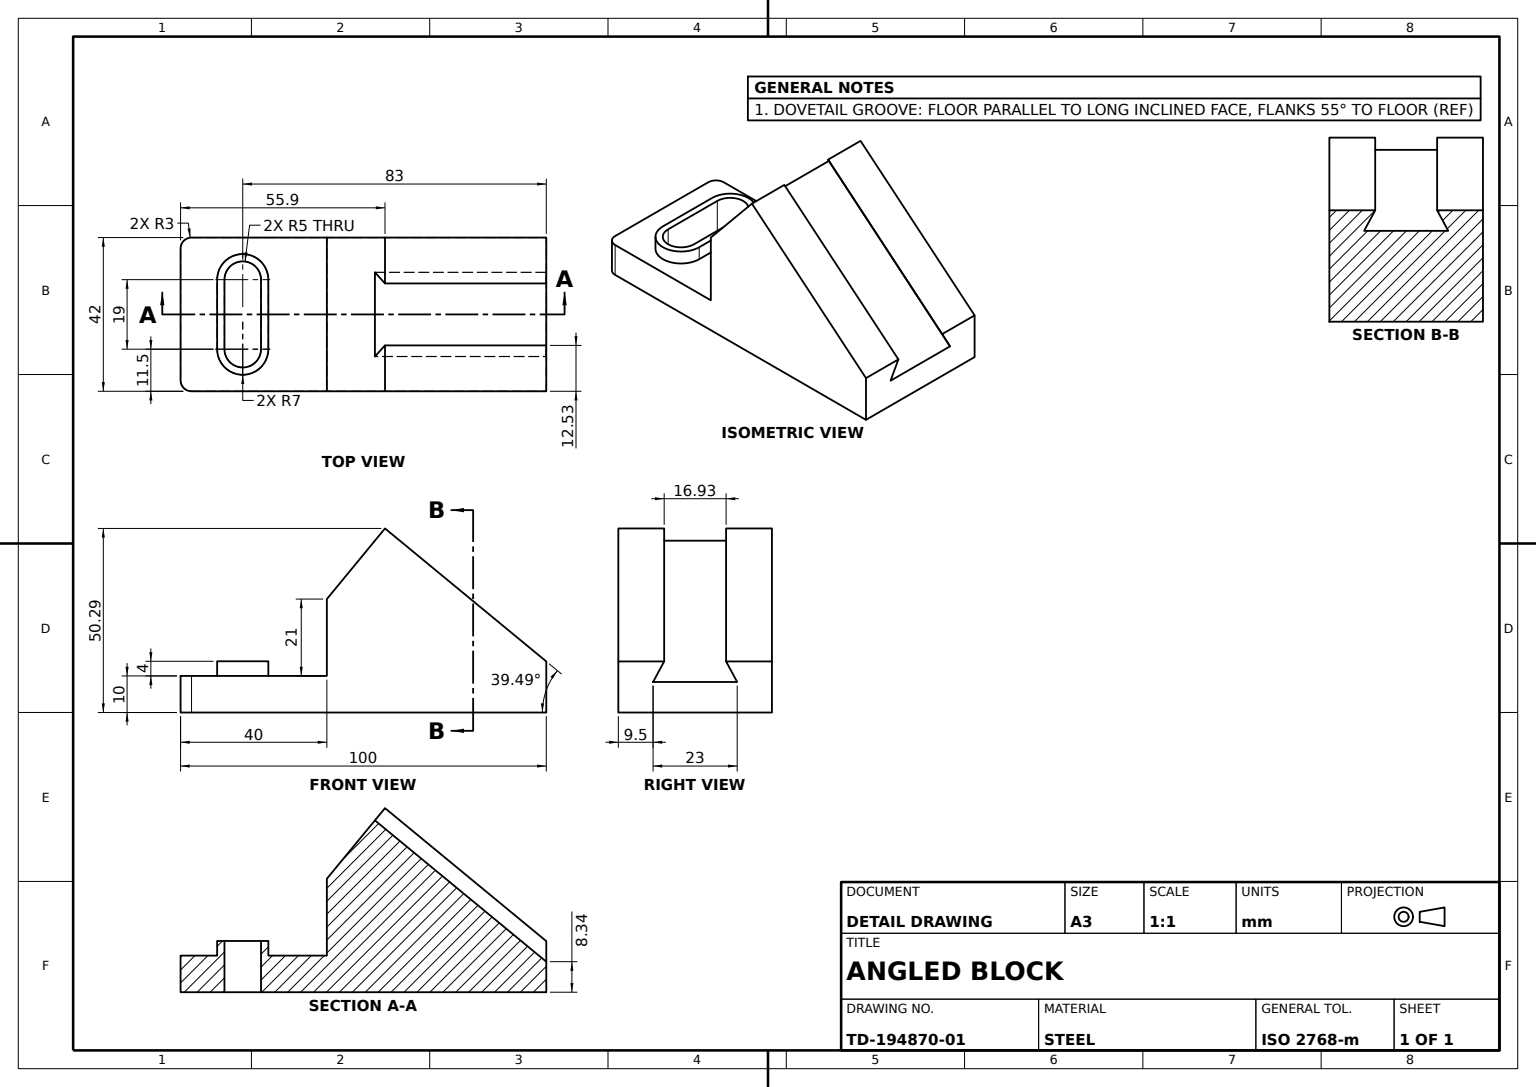
SolidWorks part; units mm, degrees
material "Plain Carbon Steel"
ref_plane "Front Plane" through (0, 0, 0) normal (0, 0, 1) x (1, 0, 0)
ref_plane "Top Plane" through (0, 0, 0) normal (0, 1, 0) x (1, 0, 0)
ref_plane "Right Plane" through (0, 0, 0) normal (1, 0, 0) x (0, 0, -1)
sketch "Base Profile Sketch" plane through (0, 0, 0) normal (0, 0, 1) x (1, 0, 0)
  line L0 (0, 0) -> (-100, 0)
  line L1 (-100, 0) -> (-100, 10)
  line L2 (-100, 10) -> (-60, 10)
  line L3 (-60, 10) -> (-60, 31)
  line L4 (-60, 31) -> (-44.1027, 50.2945)
  line L5 (-44.1027, 50.2945) -> (0, 22.736)
  line L6 (0, 22.736) -> (0, 0)
  dimension "D1" = 60
  dimension "D2" = 22.736
  dimension "D3" = 25
  dimension "D4" = 31
  dimension "D5" = 100
  dimension "D6" = 10
  dimension "D7" = 55.8973
extrude "Base Block" add sketch "Base Profile Sketch" along normal mid plane 42
sketch "Slot Boss Sketch" plane through (0, 10, 0) normal (0, 1, 0) x (1, 0, 0)
  line L0 (-88, 9.5) -> (-88, -9.5)
  line L4 (-90, 9.5) -> (-90, -9.5)
  line L5 (-76, 9.5) -> (-76, -9.5)
  line L6 (-78, 9.5) -> (-78, -9.5)
  arc A0 (-76, 9.5) -> (-90, 9.5) centre (-83, 9.5) ccw
  arc A1 (-90, -9.5) -> (-76, -9.5) centre (-83, -9.5) ccw
  arc A2 (-78, 9.5) -> (-88, 9.5) centre (-83, 9.5) ccw
  arc A3 (-88, -9.5) -> (-78, -9.5) centre (-83, -9.5) ccw
  dimension "D2" = 14
  dimension "D3" = 14
  dimension "D1" = 2
  dimension "D4" = 19
  dimension "D5" = 83
  dimension "D6" = 9.5
extrude "Slot Boss" add sketch "Slot Boss Sketch" along normal blind 4
sketch "Mounting Slot Sketch" plane through (0, 10, 0) normal (0, 1, 0) x (1, 0, 0)
  line L0 (-88, 9.5) -> (-88, -9.5)
  line L1 (-78, 9.5) -> (-78, -9.5)
  arc A0 (-78, 9.5) -> (-88, 9.5) centre (-83, 9.5) ccw
  arc A1 (-88, -9.5) -> (-78, -9.5) centre (-83, -9.5) ccw
extrude "Mounting Slot" cut sketch "Mounting Slot Sketch" against normal blind 34
sketch "Dovetail Groove Sketch" plane through (-50.9523, 41.9811, 0) normal (-0.7718, 0.6359, 0) x (0, 0, 1)
  line L0 (-11.5, 6.439) -> (-8.4663, 10.7717)
  line L2 (-11.5, 6.439) -> (11.5, 6.439)
  line L3 (11.5, 6.439) -> (8.4663, 10.7717)
  line L5 (-8.4663, 10.7717) -> (-21, 10.7717)
  line L6 (-21, 10.7717) -> (-21, 17.5472)
  line L7 (-21, 17.5472) -> (21, 17.5472)
  line L8 (21, 17.5472) -> (21, 10.7717)
  line L9 (21, 10.7717) -> (8.4663, 10.7717)
  line L10 (21, -14.2283) -> (-21, -14.2283) construction
  dimension "D1" = 23
  dimension "D2" = 11.5
  dimension "D3" = 55
  dimension "D4" = 55
  dimension "D5" = 12.5337
  dimension "D6" = 20.6674
extrude "Dovetail Groove 55°" cut sketch "Dovetail Groove Sketch" against normal blind 464
fillet "Edge Fillet R3" radius 3 2 edges at (-100, 5, -21) (-100, 5, 21)
